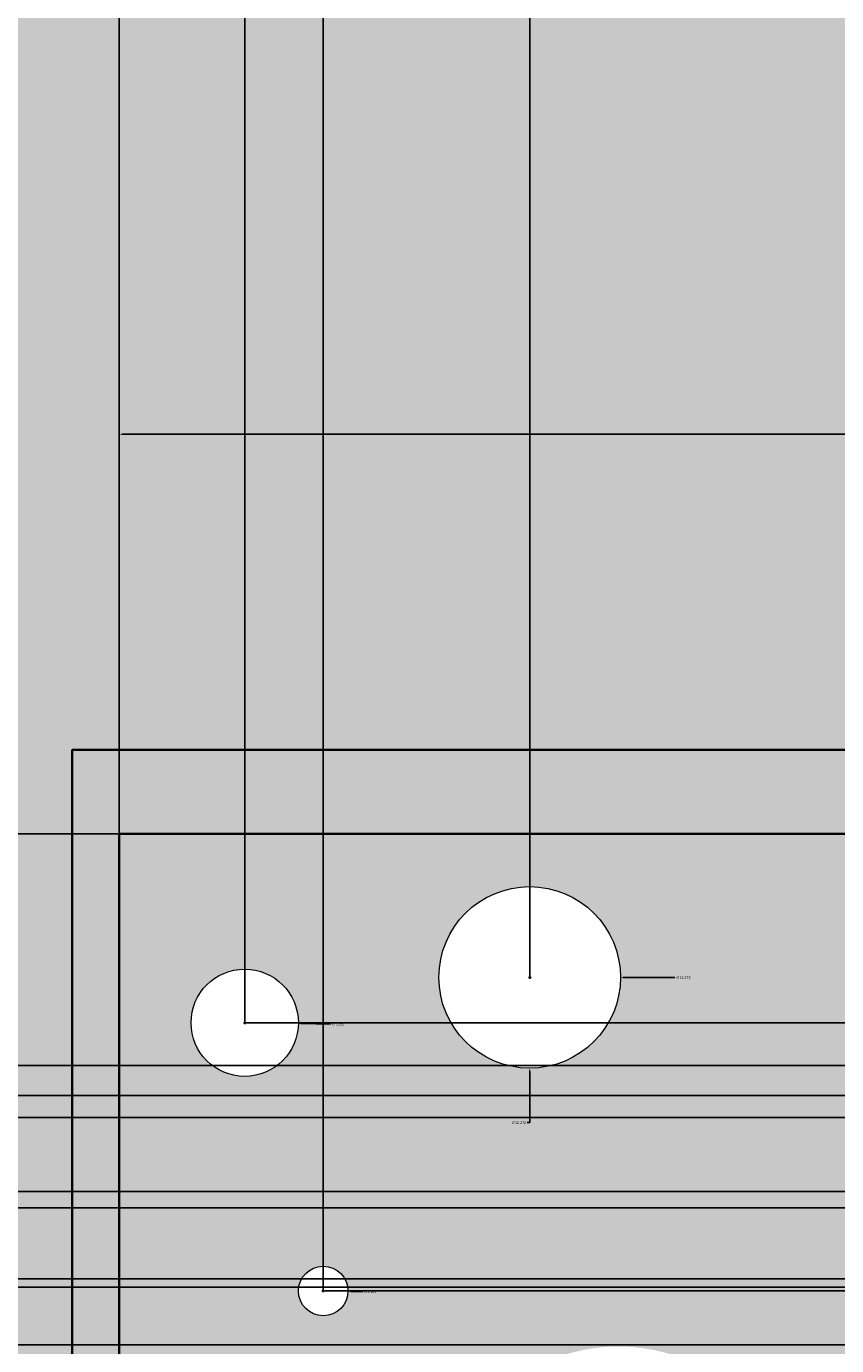
# Model space of a CAD drawing. Units: inches. Extents: x 73 to 607, y 92 to 651.
# Tile 11 of 18: x 448 to 503, y 222 to 311. Entities that reach past the tile are written whole.
import ezdxf

# ---------------------------------------------------------------- set-up
doc = ezdxf.new("R2010")
doc.units = ezdxf.units.IN
doc.header["$MEASUREMENT"] = 0
for name, color, linetype, lineweight in [('A-ANNO-DIMS', 2, 'Continuous', 18), ('A-ELEV', 7, 'Continuous', 35), ('A-ELEV-PANL', 7, 'Continuous', 18), ('A-ELEV-PATT-BKGD', 252, 'Continuous', 13), ('A-ELEV-PATT-SHAD', 8, 'Continuous', 13), ('A-ELEV-PATT-WALL', 254, 'Continuous', 13), ('A-ELEV-PATT-WOOD', 32, 'Continuous', 13)]:
    doc.layers.add(name, color=color, linetype=linetype, lineweight=lineweight)
doc.styles.get("Standard").update_dxf_attribs({"font": 'arial.ttf'})
doc.dimstyles.get("Standard").update_dxf_attribs({"dimtxt": 0.18, "dimasz": 0.18, "dimexe": 0.18, "dimexo": 0.0625, "dimgap": 0.09, "dimtad": 0, "dimtih": 1, "dimtoh": 1, "dimdec": 4, "dimzin": 0, "dimdsep": 46, "dimtxsty": 'Standard', "dimcen": 0.09, "dimadec": 0, "dimazin": 0, "dimtfac": 1, "dimtdec": 4, "dimtofl": 0, "dimtmove": 0, "dimatfit": 3, "dimfxl": 1, "dimtolj": 1, "dimtzin": 0, "dimarcsym": 0})

# ---------------------------------------------------------------- blocks, each defined once
blk = doc.blocks.new('*D17')
at = {"layer": 'A-ANNO-DIMS', "color": 0, "lineweight": -2, "transparency": 16777216}
for p, q in [((580.161, 262.302), (607.278, 262.302)), ((607.098, 262.122), (607.098, 224.164)), ((607.098, 185.842), (607.098, 223.8)), ((431.133, 185.662), (607.278, 185.662))]:
    blk.add_line(p, q, dxfattribs=at)
at = {"layer": 'A-ANNO-DIMS', "color": 0, "transparency": 16777216}
for points in [[(607.068, 262.122), (607.128, 262.122), (607.098, 262.302)], [(607.068, 185.842), (607.128, 185.842), (607.098, 185.662)]]:
    blk.add_solid(points, dxfattribs=at)
at = {"layer": 'Defpoints', "color": 0, "transparency": 16777216}
for p in [(580.098, 262.302), (607.098, 262.302), (431.07, 185.662)]:
    blk.add_point(p, dxfattribs=at)
at = {"layer": 'A-ANNO-DIMS', "color": 0, "transparency": 16777216, "insert": (607.098, 223.982), "char_height": 0.18, "attachment_point": 5}
blk.add_mtext('\\A1;76.64', dxfattribs=at)
blk = doc.blocks.new('*D39')
at = {"layer": 'A-ANNO-DIMS', "color": 0, "lineweight": -2, "transparency": 16777216}
for p, q in [((454.705, 256.695), (454.705, 283.812)), ((454.885, 283.632), (515.861, 283.632)), ((577.745, 283.632), (516.769, 283.632)), ((577.925, 256.695), (577.925, 283.812))]:
    blk.add_line(p, q, dxfattribs=at)
at = {"layer": 'A-ANNO-DIMS', "color": 0, "transparency": 16777216}
for points in [[(454.885, 283.662), (454.885, 283.602), (454.705, 283.632)], [(577.745, 283.662), (577.745, 283.602), (577.925, 283.632)]]:
    blk.add_solid(points, dxfattribs=at)
at = {"layer": 'Defpoints', "color": 0, "transparency": 16777216}
for p in [(577.925, 283.632), (454.705, 256.632), (577.925, 256.632)]:
    blk.add_point(p, dxfattribs=at)
at = {"layer": 'A-ANNO-DIMS', "color": 0, "transparency": 16777216, "insert": (516.315, 283.632), "char_height": 0.18, "attachment_point": 5}
blk.add_mtext('\\A1;123.22', dxfattribs=at)
blk = doc.blocks.new('*D40')
at = {"layer": 'A-ANNO-DIMS', "color": 0, "lineweight": -2, "transparency": 16777216}
for p, q in [((454.642, 256.632), (427.525, 256.632)), ((427.705, 256.452), (427.705, 215.899)), ((427.705, 174.982), (427.705, 215.535)), ((454.642, 174.802), (427.525, 174.802))]:
    blk.add_line(p, q, dxfattribs=at)
at = {"layer": 'A-ANNO-DIMS', "color": 0, "transparency": 16777216}
for points in [[(427.675, 256.452), (427.735, 256.452), (427.705, 256.632)], [(427.675, 174.982), (427.735, 174.982), (427.705, 174.802)]]:
    blk.add_solid(points, dxfattribs=at)
at = {"layer": 'Defpoints', "color": 0, "transparency": 16777216}
for p in [(427.705, 256.632), (454.705, 256.632), (454.705, 174.802)]:
    blk.add_point(p, dxfattribs=at)
at = {"layer": 'A-ANNO-DIMS', "color": 0, "transparency": 16777216, "insert": (427.705, 215.717), "char_height": 0.18, "attachment_point": 5}
blk.add_mtext('\\A1;81.83', dxfattribs=at)
blk = doc.blocks.new('*D64')
at = {"layer": 'A-ANNO-DIMS', "color": 0, "lineweight": -2, "transparency": 16777216}
for p, q in [((482.441, 246.834), (482.441, 247.014)), ((482.351, 246.924), (482.531, 246.924)), ((492.258, 246.924), (488.757, 246.924))]:
    blk.add_line(p, q, dxfattribs=at)
at = {"layer": 'A-ANNO-DIMS', "color": 0, "transparency": 16777216}
blk.add_solid([(488.757, 246.954), (488.757, 246.894), (488.577, 246.924)], dxfattribs=at)
at = {"layer": 'Defpoints', "color": 0, "transparency": 16777216}
for p in [(476.305, 246.924), (488.577, 246.924)]:
    blk.add_point(p, dxfattribs=at)
at = {"layer": 'A-ANNO-DIMS', "color": 0, "transparency": 16777216, "insert": (492.819, 246.924), "char_height": 0.18, "attachment_point": 5}
blk.add_mtext('\\A1;∅12.272', dxfattribs=at)
blk = doc.blocks.new('*D93')
at = {"layer": 'A-ANNO-DIMS', "color": 0, "lineweight": -2, "transparency": 16777216}
for p, q in [((349.059, 237.455), (607.278, 237.455)), ((607.098, 237.275), (607.098, 232.178)), ((607.098, 226.717), (607.098, 231.814)), ((349.059, 226.537), (607.278, 226.537))]:
    blk.add_line(p, q, dxfattribs=at)
at = {"layer": 'A-ANNO-DIMS', "color": 0, "transparency": 16777216}
for points in [[(607.068, 237.275), (607.128, 237.275), (607.098, 237.455)], [(607.068, 226.717), (607.128, 226.717), (607.098, 226.537)]]:
    blk.add_solid(points, dxfattribs=at)
at = {"layer": 'Defpoints', "color": 0, "transparency": 16777216}
for p in [(348.997, 237.455), (348.997, 226.537), (607.098, 226.537)]:
    blk.add_point(p, dxfattribs=at)
at = {"layer": 'A-ANNO-DIMS', "color": 0, "transparency": 16777216, "insert": (607.098, 231.996), "char_height": 0.18, "attachment_point": 5}
blk.add_mtext('\\A1;10.917', dxfattribs=at)
blk = doc.blocks.new('*D95')
at = {"layer": 'A-ANNO-DIMS', "color": 0, "lineweight": -2, "transparency": 16777216}
for p, q in [((363.874, 225.982), (607.278, 225.982)), ((607.098, 225.802), (607.098, 212.749)), ((607.098, 199.331), (607.098, 212.385)), ((363.319, 199.151), (607.278, 199.151))]:
    blk.add_line(p, q, dxfattribs=at)
at = {"layer": 'A-ANNO-DIMS', "color": 0, "transparency": 16777216}
for points in [[(607.068, 225.802), (607.128, 225.802), (607.098, 225.982)], [(607.068, 199.331), (607.128, 199.331), (607.098, 199.151)]]:
    blk.add_solid(points, dxfattribs=at)
at = {"layer": 'Defpoints', "color": 0, "transparency": 16777216}
for p in [(363.812, 225.982), (607.098, 225.982), (363.256, 199.151)]:
    blk.add_point(p, dxfattribs=at)
at = {"layer": 'A-ANNO-DIMS', "color": 0, "transparency": 16777216, "insert": (607.098, 212.567), "char_height": 0.18, "attachment_point": 5}
blk.add_mtext('\\A1;26.83', dxfattribs=at)
blk = doc.blocks.new('*D96')
at = {"layer": 'A-ANNO-DIMS', "color": 0, "lineweight": -2, "transparency": 16777216}
for p, q in [((360.911, 238.935), (607.278, 238.935)), ((607.098, 238.755), (607.098, 232.64)), ((607.098, 226.162), (607.098, 232.276)), ((363.874, 225.982), (607.278, 225.982))]:
    blk.add_line(p, q, dxfattribs=at)
at = {"layer": 'A-ANNO-DIMS', "color": 0, "transparency": 16777216}
for points in [[(607.068, 238.755), (607.128, 238.755), (607.098, 238.935)], [(607.068, 226.162), (607.128, 226.162), (607.098, 225.982)]]:
    blk.add_solid(points, dxfattribs=at)
at = {"layer": 'Defpoints', "color": 0, "transparency": 16777216}
for p in [(360.849, 238.935), (607.098, 238.935), (363.812, 225.982)]:
    blk.add_point(p, dxfattribs=at)
at = {"layer": 'A-ANNO-DIMS', "color": 0, "transparency": 16777216, "insert": (607.098, 232.458), "char_height": 0.18, "attachment_point": 5}
blk.add_mtext('\\A1;12.953', dxfattribs=at)
blk = doc.blocks.new('*D99')
at = {"layer": 'A-ANNO-DIMS', "color": 0, "lineweight": -2, "transparency": 16777216}
for p, q in [((373.319, 231.348), (607.278, 231.348)), ((607.098, 231.168), (607.098, 220.428)), ((607.098, 209.323), (607.098, 220.064)), ((377.023, 209.143), (607.278, 209.143))]:
    blk.add_line(p, q, dxfattribs=at)
at = {"layer": 'A-ANNO-DIMS', "color": 0, "transparency": 16777216}
for points in [[(607.068, 231.168), (607.128, 231.168), (607.098, 231.348)], [(607.068, 209.323), (607.128, 209.323), (607.098, 209.143)]]:
    blk.add_solid(points, dxfattribs=at)
at = {"layer": 'Defpoints', "color": 0, "transparency": 16777216}
for p in [(373.257, 231.348), (607.098, 231.348), (376.96, 209.143)]:
    blk.add_point(p, dxfattribs=at)
at = {"layer": 'A-ANNO-DIMS', "color": 0, "transparency": 16777216, "insert": (607.098, 220.246), "char_height": 0.18, "attachment_point": 5}
blk.add_mtext('\\A1;22.205', dxfattribs=at)
blk = doc.blocks.new('*D100')
at = {"layer": 'A-ANNO-DIMS', "color": 0, "lineweight": -2, "transparency": 16777216}
for p, q in [((382.949, 222.096), (607.278, 222.096)), ((607.098, 221.916), (607.098, 211.268)), ((607.098, 200.256), (607.098, 210.904)), ((387.579, 200.076), (607.278, 200.076))]:
    blk.add_line(p, q, dxfattribs=at)
at = {"layer": 'A-ANNO-DIMS', "color": 0, "transparency": 16777216}
for points in [[(607.068, 221.916), (607.128, 221.916), (607.098, 222.096)], [(607.068, 200.256), (607.128, 200.256), (607.098, 200.076)]]:
    blk.add_solid(points, dxfattribs=at)
at = {"layer": 'Defpoints', "color": 0, "transparency": 16777216}
for p in [(382.886, 222.096), (607.098, 222.096), (387.516, 200.076)]:
    blk.add_point(p, dxfattribs=at)
at = {"layer": 'A-ANNO-DIMS', "color": 0, "transparency": 16777216, "insert": (607.098, 211.086), "char_height": 0.18, "attachment_point": 5}
blk.add_mtext('\\A1;22.02', dxfattribs=at)
blk = doc.blocks.new('*D101')
at = {"layer": 'A-ANNO-DIMS', "color": 0, "lineweight": -2, "transparency": 16777216}
for p, q in [((382.393, 240.97), (607.278, 240.97)), ((607.098, 240.79), (607.098, 231.715)), ((607.098, 222.276), (607.098, 231.351)), ((382.949, 222.096), (607.278, 222.096))]:
    blk.add_line(p, q, dxfattribs=at)
at = {"layer": 'A-ANNO-DIMS', "color": 0, "transparency": 16777216}
for points in [[(607.068, 240.79), (607.128, 240.79), (607.098, 240.97)], [(607.068, 222.276), (607.128, 222.276), (607.098, 222.096)]]:
    blk.add_solid(points, dxfattribs=at)
at = {"layer": 'Defpoints', "color": 0, "transparency": 16777216}
for p in [(382.331, 240.97), (607.098, 240.97), (382.886, 222.096)]:
    blk.add_point(p, dxfattribs=at)
at = {"layer": 'A-ANNO-DIMS', "color": 0, "transparency": 16777216, "insert": (607.098, 231.533), "char_height": 0.18, "attachment_point": 5}
blk.add_mtext('\\A1;18.874', dxfattribs=at)
blk = doc.blocks.new('*D102')
at = {"layer": 'A-ANNO-DIMS', "color": 0, "lineweight": -2, "transparency": 16777216}
for p, q in [((382.393, 240.97), (607.278, 240.97)), ((607.098, 240.79), (607.098, 236.896)), ((607.098, 232.638), (607.098, 236.532)), ((389.616, 232.458), (607.278, 232.458))]:
    blk.add_line(p, q, dxfattribs=at)
at = {"layer": 'A-ANNO-DIMS', "color": 0, "transparency": 16777216}
for points in [[(607.068, 240.79), (607.128, 240.79), (607.098, 240.97)], [(607.068, 232.638), (607.128, 232.638), (607.098, 232.458)]]:
    blk.add_solid(points, dxfattribs=at)
at = {"layer": 'Defpoints', "color": 0, "transparency": 16777216}
for p in [(382.331, 240.97), (389.553, 232.458), (607.098, 232.458)]:
    blk.add_point(p, dxfattribs=at)
at = {"layer": 'A-ANNO-DIMS', "color": 0, "transparency": 16777216, "insert": (607.098, 236.714), "char_height": 0.18, "attachment_point": 5}
blk.add_mtext('\\A1;8.512', dxfattribs=at)
blk = doc.blocks.new('*D103')
at = {"layer": 'A-ANNO-DIMS', "color": 0, "lineweight": -2, "transparency": 16777216}
for p, q in [((454.705, 256.695), (454.705, 650.981)), ((463.18, 243.918), (463.18, 650.981)), ((454.885, 650.801), (458.548, 650.801)), ((463, 650.801), (459.337, 650.801))]:
    blk.add_line(p, q, dxfattribs=at)
at = {"layer": 'A-ANNO-DIMS', "color": 0, "transparency": 16777216}
for points in [[(454.885, 650.831), (454.885, 650.771), (454.705, 650.801)], [(463, 650.831), (463, 650.771), (463.18, 650.801)]]:
    blk.add_solid(points, dxfattribs=at)
at = {"layer": 'Defpoints', "color": 0, "transparency": 16777216}
for p in [(463.18, 650.801), (454.705, 256.632), (463.18, 243.856)]:
    blk.add_point(p, dxfattribs=at)
at = {"layer": 'A-ANNO-DIMS', "color": 0, "transparency": 16777216, "insert": (458.943, 650.801), "char_height": 0.18, "attachment_point": 5}
blk.add_mtext('\\A1;8.475', dxfattribs=at)
blk = doc.blocks.new('*D104')
at = {"layer": 'A-ANNO-DIMS', "color": 0, "lineweight": -2, "transparency": 16777216}
for p, q in [((463.18, 243.918), (463.18, 650.981)), ((468.484, 225.789), (468.484, 650.981)), ((463.36, 650.801), (465.439, 650.801)), ((468.304, 650.801), (466.225, 650.801))]:
    blk.add_line(p, q, dxfattribs=at)
at = {"layer": 'A-ANNO-DIMS', "color": 0, "transparency": 16777216}
for points in [[(463.36, 650.831), (463.36, 650.771), (463.18, 650.801)], [(468.304, 650.831), (468.304, 650.771), (468.484, 650.801)]]:
    blk.add_solid(points, dxfattribs=at)
at = {"layer": 'Defpoints', "color": 0, "transparency": 16777216}
for p in [(468.484, 650.801), (463.18, 243.856), (468.484, 225.727)]:
    blk.add_point(p, dxfattribs=at)
at = {"layer": 'A-ANNO-DIMS', "color": 0, "transparency": 16777216, "insert": (465.832, 650.801), "char_height": 0.18, "attachment_point": 5}
blk.add_mtext('\\A1;5.304', dxfattribs=at)
blk = doc.blocks.new('*D105')
at = {"layer": 'A-ANNO-DIMS', "color": 0, "lineweight": -2, "transparency": 16777216}
for p, q in [((468.484, 225.789), (468.484, 650.981)), ((482.441, 246.987), (482.441, 650.981)), ((468.664, 650.801), (475.007, 650.801)), ((482.261, 650.801), (475.917, 650.801))]:
    blk.add_line(p, q, dxfattribs=at)
at = {"layer": 'A-ANNO-DIMS', "color": 0, "transparency": 16777216}
for points in [[(468.664, 650.831), (468.664, 650.771), (468.484, 650.801)], [(482.261, 650.831), (482.261, 650.771), (482.441, 650.801)]]:
    blk.add_solid(points, dxfattribs=at)
at = {"layer": 'Defpoints', "color": 0, "transparency": 16777216}
for p in [(482.441, 650.801), (482.441, 246.924), (468.484, 225.727)]:
    blk.add_point(p, dxfattribs=at)
at = {"layer": 'A-ANNO-DIMS', "color": 0, "transparency": 16777216, "insert": (475.462, 650.801), "char_height": 0.18, "attachment_point": 5}
blk.add_mtext('\\A1;13.957', dxfattribs=at)
blk = doc.blocks.new('*D106')
at = {"layer": 'A-ANNO-DIMS', "color": 0, "lineweight": -2, "transparency": 16777216}
for p, q in [((482.441, 246.987), (482.441, 650.981)), ((509.238, 232.762), (509.238, 650.981)), ((482.621, 650.801), (495.374, 650.801)), ((509.058, 650.801), (496.304, 650.801))]:
    blk.add_line(p, q, dxfattribs=at)
at = {"layer": 'A-ANNO-DIMS', "color": 0, "transparency": 16777216}
for points in [[(482.621, 650.831), (482.621, 650.771), (482.441, 650.801)], [(509.058, 650.831), (509.058, 650.771), (509.238, 650.801)]]:
    blk.add_solid(points, dxfattribs=at)
at = {"layer": 'Defpoints', "color": 0, "transparency": 16777216}
for p in [(509.238, 650.801), (482.441, 246.924), (509.238, 232.7)]:
    blk.add_point(p, dxfattribs=at)
at = {"layer": 'A-ANNO-DIMS', "color": 0, "transparency": 16777216, "insert": (495.839, 650.801), "char_height": 0.18, "attachment_point": 5}
blk.add_mtext('\\A1;26.797', dxfattribs=at)
blk = doc.blocks.new('*D120')
at = {"layer": 'A-ANNO-DIMS', "color": 0, "lineweight": -2, "transparency": 16777216}
for p, q in [((468.546, 225.727), (607.278, 225.727)), ((607.098, 225.547), (607.098, 208.616)), ((607.098, 191.322), (607.098, 208.252)), ((469.942, 191.142), (607.278, 191.142))]:
    blk.add_line(p, q, dxfattribs=at)
at = {"layer": 'A-ANNO-DIMS', "color": 0, "transparency": 16777216}
for points in [[(607.068, 225.547), (607.128, 225.547), (607.098, 225.727)], [(607.068, 191.322), (607.128, 191.322), (607.098, 191.142)]]:
    blk.add_solid(points, dxfattribs=at)
at = {"layer": 'Defpoints', "color": 0, "transparency": 16777216}
for p in [(468.484, 225.727), (607.098, 225.727), (469.879, 191.142)]:
    blk.add_point(p, dxfattribs=at)
at = {"layer": 'A-ANNO-DIMS', "color": 0, "transparency": 16777216, "insert": (607.098, 208.434), "char_height": 0.18, "attachment_point": 5}
blk.add_mtext('\\A1;34.585', dxfattribs=at)
blk = doc.blocks.new('*D121')
at = {"layer": 'A-ANNO-DIMS', "color": 0, "lineweight": -2, "transparency": 16777216}
for p, q in [((463.243, 243.856), (607.278, 243.856)), ((607.098, 243.676), (607.098, 234.973)), ((607.098, 225.907), (607.098, 234.609)), ((468.546, 225.727), (607.278, 225.727))]:
    blk.add_line(p, q, dxfattribs=at)
at = {"layer": 'A-ANNO-DIMS', "color": 0, "transparency": 16777216}
for points in [[(607.068, 243.676), (607.128, 243.676), (607.098, 243.856)], [(607.068, 225.907), (607.128, 225.907), (607.098, 225.727)]]:
    blk.add_solid(points, dxfattribs=at)
at = {"layer": 'Defpoints', "color": 0, "transparency": 16777216}
for p in [(463.18, 243.856), (607.098, 243.856), (468.484, 225.727)]:
    blk.add_point(p, dxfattribs=at)
at = {"layer": 'A-ANNO-DIMS', "color": 0, "transparency": 16777216, "insert": (607.098, 234.791), "char_height": 0.18, "attachment_point": 5}
blk.add_mtext('\\A1;18.13', dxfattribs=at)
blk = doc.blocks.new('*D154')
at = {"layer": 'A-ANNO-DIMS', "color": 0, "lineweight": -2, "transparency": 16777216}
for p, q in [((463.09, 243.856), (463.27, 243.856)), ((463.18, 243.766), (463.18, 243.946)), ((468.981, 243.767), (466.986, 243.798))]:
    blk.add_line(p, q, dxfattribs=at)
at = {"layer": 'A-ANNO-DIMS', "color": 0, "transparency": 16777216}
blk.add_solid([(466.986, 243.828), (466.985, 243.768), (466.806, 243.8)], dxfattribs=at)
at = {"layer": 'Defpoints', "color": 0, "transparency": 16777216}
for p in [(459.555, 243.912), (466.806, 243.8)]:
    blk.add_point(p, dxfattribs=at)
at = {"layer": 'A-ANNO-DIMS', "color": 0, "transparency": 16777216, "insert": (469.472, 243.767), "char_height": 0.18, "attachment_point": 5}
blk.add_mtext('\\A1;∅7.252', dxfattribs=at)
blk = doc.blocks.new('*D155')
at = {"layer": 'A-ANNO-DIMS', "color": 0, "lineweight": -2, "transparency": 16777216}
for p, q in [((482.441, 246.834), (482.441, 247.014)), ((482.351, 246.924), (482.531, 246.924)), ((482.44, 237.106), (482.44, 240.608)), ((482.26, 237.106), (482.44, 237.106))]:
    blk.add_line(p, q, dxfattribs=at)
at = {"layer": 'A-ANNO-DIMS', "color": 0, "transparency": 16777216}
blk.add_solid([(482.41, 240.608), (482.47, 240.608), (482.44, 240.788)], dxfattribs=at)
at = {"layer": 'Defpoints', "color": 0, "transparency": 16777216}
for p in [(482.441, 253.06), (482.44, 240.788)]:
    blk.add_point(p, dxfattribs=at)
at = {"layer": 'A-ANNO-DIMS', "color": 0, "transparency": 16777216, "insert": (481.699, 237.106), "char_height": 0.18, "attachment_point": 5}
blk.add_mtext('\\A1;∅12.272', dxfattribs=at)
blk = doc.blocks.new('*D160')
at = {"layer": 'A-ANNO-DIMS', "color": 0, "lineweight": -2, "transparency": 16777216}
for p, q in [((468.394, 225.727), (468.574, 225.727)), ((468.484, 225.637), (468.484, 225.817)), ((471.161, 225.682), (470.337, 225.696))]:
    blk.add_line(p, q, dxfattribs=at)
at = {"layer": 'A-ANNO-DIMS', "color": 0, "transparency": 16777216}
blk.add_solid([(470.338, 225.726), (470.337, 225.666), (470.157, 225.699)], dxfattribs=at)
at = {"layer": 'Defpoints', "color": 0, "transparency": 16777216}
for p in [(466.811, 225.755), (470.157, 225.699)]:
    blk.add_point(p, dxfattribs=at)
at = {"layer": 'A-ANNO-DIMS', "color": 0, "transparency": 16777216, "insert": (471.653, 225.682), "char_height": 0.18, "attachment_point": 5}
blk.add_mtext('\\A1;∅3.347', dxfattribs=at)

msp = doc.modelspace()

# ---------------------------------------------------------------- hatches: boundary and pattern name
at = {"layer": 'A-ELEV-PATT-BKGD'}
h = msp.add_hatch(color=256, dxfattribs=at)
h.dxf.hatch_style = 1
h.paths.add_polyline_path([(321.3008, 479.2042), (312.3008, 479.2042), (312.3008, 478.7576), (312.3008, 412.636), (321.3008, 412.636)])
h.paths.add_polyline_path([(312.3008, 504.7576), (256.4726, 504.7576), (256.4726, 503.4576), (312.3008, 503.4576)], flags=17)
h.paths.add_polyline_path([(321.3008, 543.1576), (321.3008, 552.1576), (320.3257, 552.1576), (312.3008, 552.1576), (256.4726, 552.1576), (256.4726, 543.1576), (312.3008, 543.1576), (312.3008, 479.2042), (321.3008, 479.2042)])
h.paths.add_polyline_path([(451.5214, 412.636), (256.4726, 412.636), (256.4726, 403.636), (442.5214, 403.636), (442.5214, 320.2042), (206.1343, 320.2042), (206.1343, 320.9135), (206.1343, 403.636), (256.4726, 403.636), (256.4726, 412.636), (201.6343, 412.636), (201.6343, 320.9135), (201.6343, 320.2042), (201.6343, 311.2042), (256.4726, 311.2042), (451.5214, 311.2042)])
h.paths.add_polyline_path([(431.07, 258.6914), (369.5339, 258.6914), (369.5339, 247.4054), (396.692, 247.4054), (425.07, 247.4054), (425.07, 194.7312), (396.692, 194.6197), (396.692, 194.5366), (369.5339, 194.5366), (369.5339, 185.6619), (431.07, 185.6619)])
h.paths.add_polyline_path([(580.0983, 262.3024), (451.5214, 262.3024), (451.5214, 143.2042), (580.0983, 143.2042)])
h.paths.add_polyline_path([(454.7049, 174.802), (454.7049, 256.6321), (577.9249, 256.6321), (577.9249, 174.802)], flags=16)
h.paths.add_polyline_path([(465.9716, 191.1416, -1), (473.7874, 191.1416, -1)], flags=0)
h.paths.add_polyline_path([(490.5373, 181.6586, -1), (494.9999, 181.6586, -1)], flags=0)
h.paths.add_polyline_path([(476.2996, 209.8287, -1), (500.5844, 209.8287, -1)], flags=0)
h.paths.add_polyline_path([(505.3326, 194.7675, -1), (512.5843, 194.7675, -1)], flags=0)
h.paths.add_polyline_path([(520.9613, 186.679, -1), (526.544, 186.679, -1)], flags=0)
h.paths.add_polyline_path([(466.8103, 225.7267, -1), (470.1573, 225.7267, -1)], flags=0)
h.paths.add_polyline_path([(527.1059, 203.6926, -1), (536.0311, 203.6926, -1)], flags=0)
h.paths.add_polyline_path([(504.775, 232.6995, -1), (513.7002, 232.6995, -1)], flags=0)
h.paths.add_polyline_path([(546.9241, 183.611, -1), (554.7336, 183.611, -1)], flags=0)
h.paths.add_polyline_path([(459.5544, 243.856, -1), (466.8061, 243.856, -1)], flags=0)
h.paths.add_polyline_path([(476.3045, 246.924, -1), (488.5767, 246.924, -1)], flags=0)
h.paths.add_polyline_path([(529.9044, 226.8424, -1), (556.68, 226.8424, -1)], flags=0)
h.paths.add_polyline_path([(554.1814, 203.9716, -1), (561.4331, 203.9716, -1)], flags=0)
h.paths.add_polyline_path([(567.8561, 193.3729, -1), (570.6475, 193.3729, -1)], flags=0)
h.paths.add_polyline_path([(522.3584, 250.271, -1), (525.7053, 250.271, -1)], flags=0)
h.paths.add_polyline_path([(561.9965, 245.2506, -1), (567.5748, 245.2506, -1)], flags=0)
h.paths.add_polyline_path([(347.8686, 194.5366), (341.8686, 194.5366), (341.8686, 194.5452), (314.0144, 194.5452), (314.0144, 188.5452), (347.8686, 188.5452)])
h.paths.add_polyline_path([(347.8686, 253.4054), (314.0144, 253.4054), (314.0144, 247.4054), (341.8686, 247.4054), (347.8686, 247.4054)])
h.paths.add_polyline_path([(304.3559, 253.4054), (298.3559, 253.4054), (298.3559, 188.5452), (304.3559, 188.5452)])
h.paths.add_polyline_path([(450.6603, 552.1576), (369.9727, 552.1576), (369.9727, 479.2042), (374.4727, 479.2042), (374.4727, 547.6576), (446.1603, 547.6576), (446.1603, 479.2042), (450.6603, 479.2042)])
h.paths.add_polyline_path([(374.4727, 479.2042), (369.9727, 479.2042), (369.9727, 465.0632), (374.4727, 465.0632)])
h.paths.add_polyline_path([(450.6603, 479.2042), (446.1603, 479.2042), (446.1603, 465.0632), (450.6603, 465.0632)])
h.paths.add_polyline_path([(256.4726, 281.6039), (109.0983, 281.6039), (100.0983, 281.6039), (100.0983, 167.2042), (100.0983, 143.2042), (109.0983, 143.2042), (109.0983, 167.2042), (109.0983, 272.6039), (256.4726, 272.6039)])
at = {"layer": 'A-ELEV-PATT-SHAD'}
h = msp.add_hatch(color=256, dxfattribs=at)
h.dxf.hatch_style = 1
h.paths.add_polyline_path([(451.5214, 412.636), (256.4726, 412.636), (256.4726, 403.636), (442.5214, 403.636), (442.5214, 320.2042), (206.1343, 320.2042), (206.1343, 320.9135), (206.1343, 403.636), (256.4726, 403.636), (256.4726, 412.636), (201.6343, 412.636), (201.6343, 320.9135), (201.6343, 320.2042), (201.6343, 311.2042), (256.4726, 311.2042), (451.5214, 311.2042)])
h.paths.add_polyline_path([(580.0983, 262.3024), (451.5214, 262.3024), (451.5214, 143.2042), (580.0983, 143.2042)])
h.paths.add_polyline_path([(454.7049, 174.802), (454.7049, 256.6321), (577.9249, 256.6321), (577.9249, 174.802)], flags=16)
h.paths.add_polyline_path([(465.9716, 191.1416, -1), (473.7874, 191.1416, -1)], flags=0)
h.paths.add_polyline_path([(490.5373, 181.6586, -1), (494.9999, 181.6586, -1)], flags=0)
h.paths.add_polyline_path([(476.2996, 209.8287, -1), (500.5844, 209.8287, -1)], flags=0)
h.paths.add_polyline_path([(505.3326, 194.7675, -1), (512.5843, 194.7675, -1)], flags=0)
h.paths.add_polyline_path([(520.9613, 186.679, -1), (526.544, 186.679, -1)], flags=0)
h.paths.add_polyline_path([(466.8103, 225.7267, -1), (470.1573, 225.7267, -1)], flags=0)
h.paths.add_polyline_path([(527.1059, 203.6926, -1), (536.0311, 203.6926, -1)], flags=0)
h.paths.add_polyline_path([(459.5544, 243.856, -1), (466.8061, 243.856, -1)], flags=0)
h.paths.add_polyline_path([(504.775, 232.6995, -1), (513.7002, 232.6995, -1)], flags=0)
h.paths.add_polyline_path([(476.3045, 246.924, -1), (488.5767, 246.924, -1)], flags=0)
h.paths.add_polyline_path([(546.9241, 183.611, -1), (554.7336, 183.611, -1)], flags=0)
h.paths.add_polyline_path([(529.9044, 226.8424, -1), (556.68, 226.8424, -1)], flags=0)
h.paths.add_polyline_path([(554.1814, 203.9716, -1), (561.4331, 203.9716, -1)], flags=0)
h.paths.add_polyline_path([(522.3584, 250.271, -1), (525.7053, 250.271, -1)], flags=0)
h.paths.add_polyline_path([(567.8561, 193.3729, -1), (570.6475, 193.3729, -1)], flags=0)
h.paths.add_polyline_path([(561.9965, 245.2506, -1), (567.5748, 245.2506, -1)], flags=0)
h.paths.add_polyline_path([(431.07, 258.6914), (369.5339, 258.6914), (369.5339, 247.4054), (396.692, 247.4054), (425.07, 247.4054), (425.07, 194.7312), (396.692, 194.6197), (396.692, 194.5366), (369.5339, 194.5366), (369.5339, 185.6619), (431.07, 185.6619)])
h.paths.add_polyline_path([(347.8686, 253.4054), (314.0144, 253.4054), (314.0144, 247.4054), (341.8686, 247.4054), (347.8686, 247.4054)])
h.paths.add_polyline_path([(304.3559, 253.4054), (298.3559, 253.4054), (298.3559, 188.5452), (304.3559, 188.5452)])
h.paths.add_polyline_path([(347.8686, 194.5366), (341.8686, 194.5366), (341.8686, 194.5452), (314.0144, 194.5452), (314.0144, 188.5452), (347.8686, 188.5452)])
at = {"layer": 'A-ELEV-PATT-WALL'}
h = msp.add_hatch(color=256, dxfattribs=at)
h.dxf.hatch_style = 1
h.paths.add_polyline_path([(509.9692, 483.857), (450.6603, 483.857), (450.6603, 465.0632), (446.1603, 465.0632), (446.1603, 484.2142), (374.4727, 484.2142), (374.4727, 465.0632), (369.9727, 465.0632), (369.9727, 484.2142), (321.3008, 484.2142), (321.3008, 412.636), (451.5214, 412.636), (451.5214, 311.2042), (314.0144, 311.2042), (314.0144, 253.4054), (347.8686, 253.4054), (347.8686, 247.4054), (369.5339, 247.4054), (369.5339, 258.6914), (431.07, 258.6914), (431.07, 185.6619), (369.5339, 185.6619), (369.5339, 194.5366), (347.8686, 194.5366), (347.8686, 188.5452), (314.0144, 188.5452), (314.0144, 143.2042), (451.5214, 143.2042), (451.5214, 262.3024), (580.0983, 262.3024), (580.0983, 311.2042), (509.9692, 311.2042)])
h.paths.add_polyline_path([(304.3559, 311.2042), (256.4726, 311.2042), (256.4726, 167.2042), (256.4726, 143.2042), (304.3559, 143.2042), (304.3559, 188.5452), (298.3559, 188.5452), (298.3559, 253.4054), (304.3559, 253.4054)])
at = {"layer": 'A-ELEV-PATT-WOOD'}
h = msp.add_hatch(color=256, dxfattribs=at)
h.dxf.hatch_style = 1
h.paths.add_polyline_path([(577.9249, 256.6321), (454.7049, 256.6321), (454.7049, 174.802), (577.9249, 174.802)])
h.paths.add_polyline_path([(476.2996, 209.8287, -1), (500.5844, 209.8287, -1)], flags=16)
h.paths.add_polyline_path([(473.7874, 191.1416, -1), (465.9716, 191.1416, -1)], flags=16)
h.paths.add_polyline_path([(466.8103, 225.7267, -1), (470.1573, 225.7267, -1)], flags=16)
h.paths.add_polyline_path([(459.5544, 243.856, -1), (466.8061, 243.856, -1)], flags=16)
h.paths.add_polyline_path([(494.9999, 181.6586, -1), (490.5373, 181.6586, -1)], flags=16)
h.paths.add_polyline_path([(476.3045, 246.924, -1), (488.5767, 246.924, -1)], flags=16)
h.paths.add_polyline_path([(512.5843, 194.7675, -1), (505.3326, 194.7675, -1)], flags=16)
h.paths.add_polyline_path([(504.775, 232.6995, -1), (513.7002, 232.6995, -1)], flags=16)
h.paths.add_polyline_path([(526.544, 186.679, -1), (520.9613, 186.679, -1)], flags=16)
h.paths.add_polyline_path([(536.0311, 203.6926, -1), (527.1059, 203.6926, -1)], flags=16)
h.paths.add_polyline_path([(529.9044, 226.8424, -1), (556.68, 226.8424, -1)], flags=16)
h.paths.add_polyline_path([(522.3584, 250.271, -1), (525.7053, 250.271, -1)], flags=16)
h.paths.add_polyline_path([(554.7336, 183.611, -1), (546.9241, 183.611, -1)], flags=16)
h.paths.add_polyline_path([(561.4331, 203.9716, -1), (554.1814, 203.9716, -1)], flags=16)
h.paths.add_polyline_path([(561.9965, 245.2506, -1), (567.5748, 245.2506, -1)], flags=16)
h.paths.add_polyline_path([(570.6475, 193.3729, -1), (567.8561, 193.3729, -1)], flags=16)

# ---------------------------------------------------------------- linework, layer by layer
at = {"layer": 'A-ELEV'}
for points in [[(580.0983, 143.2042), (451.5214, 143.2042), (451.5214, 262.3024), (580.0983, 262.3024)], [(454.7049, 256.6321), (577.9249, 256.6321), (577.9249, 174.802), (454.7049, 174.802)]]:
    msp.add_lwpolyline(points, close=True, dxfattribs=at)
at = {"layer": 'A-ELEV-PANL'}
for centre, radius in [((482.4406, 246.924), 6.1361), ((463.1802, 243.856), 3.6259), ((468.4838, 225.7267), 1.6735)]:
    msp.add_circle(centre, radius, dxfattribs=at)

# ---------------------------------------------------------------- dimensions: what is measured, and where the dimension line sits
at = {"layer": 'A-ANNO-DIMS'}
for base, p1, p2, override, picture, middle in [((463.1802, 650.801), (454.7049, 256.6321), (463.1802, 243.856), {"dimdec": 3, "dimlfac": 1, "dimrnd": 0, "dimzin": 0, "dimdsep": 46, "dimlunit": 2}, '*D103', (458.9425, 650.801)), ((468.4838, 650.801), (463.1802, 243.856), (468.4838, 225.7267), {"dimdec": 3, "dimlfac": 1, "dimrnd": 0, "dimzin": 0, "dimdsep": 46, "dimlunit": 2}, '*D104', (465.832, 650.801)), ((482.4406, 650.801), (468.4838, 225.7267), (482.4406, 246.924), {"dimdec": 3, "dimlfac": 1, "dimrnd": 0, "dimzin": 0, "dimdsep": 46, "dimlunit": 2}, '*D105', (475.4622, 650.801)), ((509.2376, 650.801), (482.4406, 246.924), (509.2376, 232.6995), {"dimdec": 3, "dimlfac": 1, "dimrnd": 0, "dimzin": 0, "dimdsep": 46, "dimlunit": 2}, '*D106', (495.8391, 650.801)), ((577.9249, 283.6321), (454.7049, 256.6321), (577.9249, 256.6321), {"dimdec": 2, "dimlfac": 1, "dimrnd": 0, "dimzin": 0, "dimdsep": 46, "dimlunit": 2}, '*D39', (516.3149, 283.6321))]:
    dim = msp.add_linear_dim(base=base, p1=p1, p2=p2, dimstyle='Standard', override=override, dxfattribs=at)
    dim.commit()
    dim.dimension.update_dxf_attribs({"geometry": picture, "text_midpoint": middle})
for base, p1, p2, override, picture, middle in [((607.0983, 262.3024), (431.07, 185.6619), (580.0983, 262.3024), {"dimdec": 2, "dimlfac": 1, "dimrnd": 0, "dimzin": 0, "dimdsep": 46, "dimlunit": 2}, '*D17', (607.0983, 223.9821)), ((427.7049, 256.6321), (454.7049, 174.802), (454.7049, 256.6321), {"dimdec": 2, "dimlfac": 1, "dimrnd": 0, "dimzin": 0, "dimdsep": 46, "dimlunit": 2}, '*D40', (427.7049, 215.7171)), ((607.0983, 243.856), (468.4838, 225.7267), (463.1802, 243.856), {"dimdec": 2, "dimlfac": 1, "dimrnd": 0, "dimzin": 0, "dimdsep": 46, "dimlunit": 2}, '*D121', (607.0983, 234.7914)), ((607.0983, 240.9703), (382.8864, 222.0962), (382.3308, 240.9703), {"dimdec": 3, "dimlfac": 1, "dimrnd": 0, "dimzin": 0, "dimdsep": 46, "dimlunit": 2}, '*D101', (607.0983, 231.5333)), ((607.0983, 232.4585), (382.3308, 240.9703), (389.5532, 232.4585), {"dimdec": 3, "dimlfac": 1, "dimrnd": 0, "dimzin": 0, "dimdsep": 46, "dimlunit": 2}, '*D102', (607.0983, 236.7144)), ((607.0983, 238.9349), (363.8119, 225.982), (360.8489, 238.9349), {"dimdec": 3, "dimlfac": 1, "dimrnd": 0, "dimzin": 0, "dimdsep": 46, "dimlunit": 2}, '*D96', (607.0983, 232.4585)), ((607.0983, 226.5372), (348.9968, 237.4546), (348.9968, 226.5372), {"dimdec": 3, "dimlfac": 1, "dimrnd": 0, "dimzin": 0, "dimdsep": 46, "dimlunit": 2}, '*D93', (607.0983, 231.9959)), ((607.0983, 231.3482), (376.9603, 209.1433), (373.2566, 231.3482), {"dimdec": 3, "dimlfac": 1, "dimrnd": 0, "dimzin": 0, "dimdsep": 46, "dimlunit": 2}, '*D99', (607.0983, 220.2458)), ((607.0983, 225.982), (363.2564, 199.1512), (363.8119, 225.982), {"dimdec": 2, "dimlfac": 1, "dimrnd": 0, "dimzin": 0, "dimdsep": 46, "dimlunit": 2}, '*D95', (607.0983, 212.5666)), ((607.0983, 225.7267), (469.8795, 191.1416), (468.4838, 225.7267), {"dimdec": 3, "dimlfac": 1, "dimrnd": 0, "dimzin": 0, "dimdsep": 46, "dimlunit": 2}, '*D120', (607.0983, 208.4342)), ((607.0983, 222.0962), (387.5161, 200.0764), (382.8864, 222.0962), {"dimdec": 2, "dimlfac": 1, "dimrnd": 0, "dimzin": 0, "dimdsep": 46, "dimlunit": 2}, '*D100', (607.0983, 211.0863))]:
    dim = msp.add_linear_dim(base=base, p1=p1, p2=p2, angle=90, dimstyle='Standard', override=override, dxfattribs=at)
    dim.commit()
    dim.dimension.update_dxf_attribs({"geometry": picture, "text_midpoint": middle})
for p1, p2, picture, middle in [((482.4412, 253.0601), (482.44, 240.788), '*D155', (481.699, 237.1063)), ((476.3045, 246.9241), (488.5767, 246.924), '*D64', (492.2583, 246.924)), ((459.5548, 243.9116), (466.8057, 243.8004), '*D154', (468.9809, 243.767)), ((466.8106, 225.7547), (470.157, 225.6987), '*D160', (471.161, 225.6819))]:
    dim = msp.add_diameter_dim_2p(p1=p1, p2=p2, dimstyle='Standard', override={"dimdec": 3, "dimlfac": 1, "dimrnd": 0, "dimzin": 0, "dimdsep": 46, "dimlunit": 2}, dxfattribs=at)
    dim.commit()
    dim.dimension.update_dxf_attribs({"geometry": picture, "text_midpoint": middle, "dimtype": 163})

doc.saveas('drawing.dxf')
